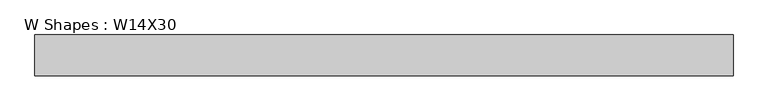
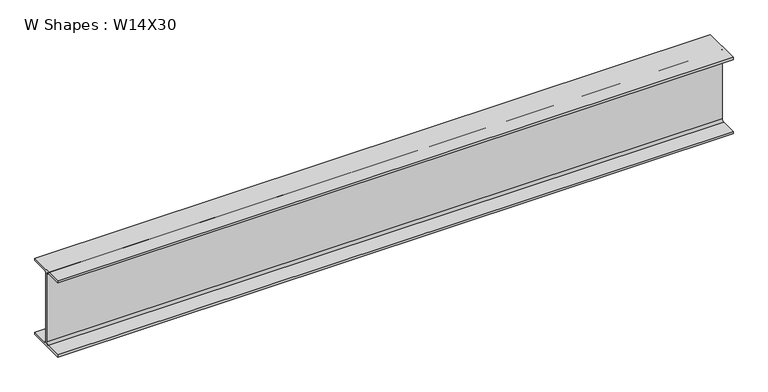
"""IFC4 building model written with IfcOpenShell, lengths in millimetres: beam geometry, W Shapes : W14X30."""

from ifc_helpers import new_model, si_unit, point, frame, frame_2d, origin, place, context, project, spatial, polyline, circle_curve, trimmed, segment, composite_curve, outline, extrude, source, transform, mapped, element, save


def w_shapes_w14x30_b6c746c8(model_context):
    return source(origin(), model_context, "Body", "SweptSolid", [
        extrude(outline(composite_curve([segment(polyline([(85.471, -165.481), (85.471, -175.26), (-85.471, -175.26), (-85.471, -165.481), (-13.589, -165.481)]), True, "CONTINUOUS"), segment(trimmed(circle_curve(frame_2d((-13.589, -155.321)), 10.16), [point((-13.589, -165.481))], [point((-3.429, -155.321))], True, "CARTESIAN"), True, "CONTINUOUS"), segment(polyline([(-3.429, -155.321), (-3.429, 155.321)]), True, "CONTINUOUS"), segment(trimmed(circle_curve(frame_2d((-13.589, 155.321)), 10.16), [point((-3.429, 155.321))], [point((-13.589, 165.481))], True, "CARTESIAN"), True, "CONTINUOUS"), segment(polyline([(-13.589, 165.481), (-85.471, 165.481), (-85.471, 175.26), (85.471, 175.26), (85.471, 165.481), (13.589, 165.481)]), True, "CONTINUOUS"), segment(trimmed(circle_curve(frame_2d((13.589, 155.321)), 10.16), [point((13.589, 165.481))], [point((3.429, 155.321))], True, "CARTESIAN"), True, "CONTINUOUS"), segment(polyline([(3.429, 155.321), (3.429, -155.321)]), True, "CONTINUOUS"), segment(trimmed(circle_curve(frame_2d((13.589, -155.321)), 10.16), [point((3.429, -155.321))], [point((13.589, -165.481))], True, "CARTESIAN"), True, "CONTINUOUS"), segment(polyline([(13.589, -165.481), (85.471, -165.481)]), True, "CONTINUOUS")], self_intersect=False)), frame((-1546.4459375, 0.0, 0.0), z_axis=(1.0, 0.0, 0.0), x_axis=(0.0, 1.0, 0.0)), (0.0, 0.0, 1.0), 2933.2566267),
    ])


if __name__ == "__main__":
    model = new_model("IFC4")
    model_context = context("Model", 3, world=origin())
    ifc_project = project(units=[si_unit("LENGTHUNIT", "METRE", prefix="MILLI")], contexts=[model_context])
    site = spatial("IfcSite", under=ifc_project)
    building = spatial("IfcBuilding", under=site)
    placement = place(None, origin())
    w_shapes_w14x30_shape = w_shapes_w14x30_b6c746c8(model_context)
    element("IfcBeam", 1, ObjectType="W Shapes : W14X30", at=placement, inside=building, context=model_context, shape_type="MappedRepresentation", body=[
        mapped(w_shapes_w14x30_shape, transform((0.0, 0.0, 0.0), x_axis=(1.0, 0.0, 0.0), y_axis=(0.0, 1.0, 0.0), z_axis=(0.0, 0.0, 1.0))),
    ])
    save(model, "model.ifc")

# Revit data of these elements
# Type "W Shapes : W14X30"
#   Section Name Key = "W14X30"
#   Width = 6.730"
#   Web Thickness = 0.270"
#   Web Fillet = 0.400"
#   Warping Constant = 887.00 in⁶
#   Torsional Moment of Inertia = 0.38 in⁴
#   Section Area = 8.85 in²
#   Plastic Modulus weak axis = 8.99 in³
#   Plastic Modulus strong axis = 47.30 in³
#   Perimeter = 4.441 ft²/ft
#   Nominal Weight = 30.00 lbf/ft
#   Moment of Inertia weak axis = 19.60 in⁴
#   Moment of Inertia strong axis = 291.00 in⁴
#   Height = 13.800"
#   Flange Thickness = 0.385"
#   Elastic Modulus weak axis = 5.82 in³
#   Elastic Modulus strong axis = 42.00 in³
#   Clear Web Height = 0' - 11 5/8"
#   Centroid Vertical = 6.900"
#   Centroid Horizontal = 3.365"
#   Bolt Spacing = 0' - 3 1/2"
#   Length [instance default] = 1524 mm
#   Structural Material [instance default] = Steel ASTM A992
#   Principal Axes Angle = 0
# Element 1 (IfcBeam, "W Shapes : W14X30")
#   Length = 3871.876 mm
#   Materials on its faces: "Steel ASTM A992"
# Materials
#   "Steel ASTM A992": class "Metal", colour RGB 199 199 199, transparency 0, Description = "Structural steel 50ksi", Cost = 0
